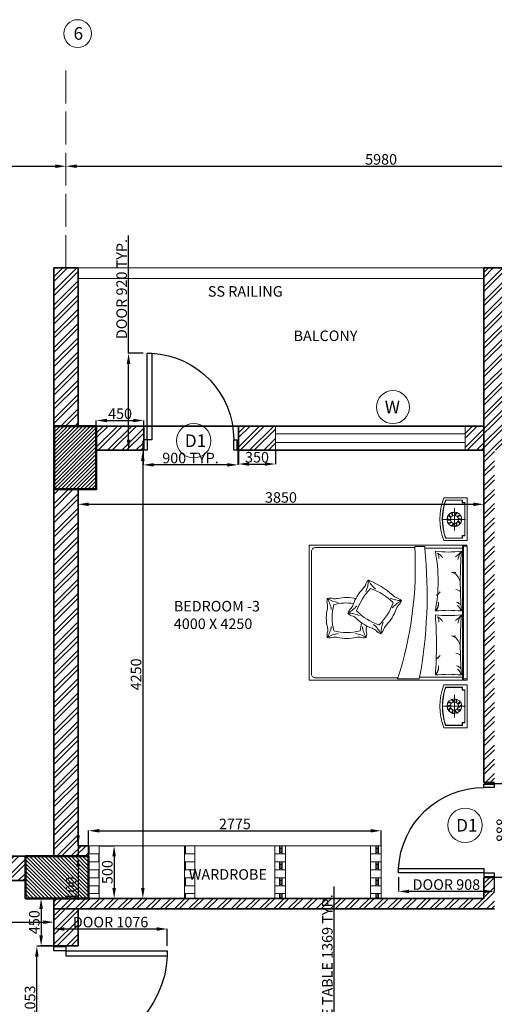
# Model space of a CAD drawing. Units: millimetres. Extents: x -3326 to 29338, y -16792 to 6002.
# Tile 19 of 21: x 16958 to 21462, y -3388 to 5950. Entities that reach past the tile are written whole.
import ezdxf

# ---------------------------------------------------------------- set-up
doc = ezdxf.new("R2010")
doc.units = ezdxf.units.MM
doc.header["$PDMODE"] = 35
doc.header["$PDSIZE"] = 5
doc.linetypes.add('ACAD_ISO04W100', pattern=[30, 24, -3, 0, -3])
for name, color, linetype, lineweight in [('A-ANNO-DIMS', 2, 'Continuous', 13), ('A-ANNO-SYMB', 7, 'Continuous', 18), ('A-AREA-IDEN', 7, 'Continuous', 18), ('A-COLS', 1, 'Continuous', 50), ('A-COLS-PATT', 251, 'Continuous', 13), ('A-DOOR', 3, 'Continuous', 25), ('A-FLOR-CASE', 30, 'Continuous', 18), ('A-FLOR-CASE-PATT', 252, 'Continuous', 13), ('A-FLOR-RAIL', 8, 'Continuous', 20), ('A-GLAZ', 4, 'Continuous', 18), ('A-GRID', 8, 'ACAD_ISO04W100', 13), ('A-GRID-IDEN', 7, 'Continuous', 18), ('A-WALL', 7, 'Continuous', 35), ('A-WALL-PATT', 252, 'Continuous', 13), ('furn', 28, 'Continuous', 18), ('txt', 7, 'Continuous', 18)]:
    doc.layers.add(name, color=color, linetype=linetype, lineweight=lineweight)
doc.styles.get("Standard").update_dxf_attribs({"font": 'arial.ttf'})
doc.dimstyles.new('ISO-25', dxfattribs={"dimtxt": 100, "dimasz": 100, "dimexe": 1.25, "dimexo": 0.625, "dimtad": 1, "dimtxsty": 'Standard', "dimcen": 2.5, "dimadec": 0, "dimazin": 0, "dimtfac": 1, "dimtmove": 0, "dimatfit": 3, "dimfxl": 1, "dimarcsym": 0})
pattern_1 = [(45, (-10476.65, 1e-12), (-67.35192, 67.35192), []), (45, (-10431.74, 1e-12), (-67.35192, 67.35192), [])]

# ---------------------------------------------------------------- blocks, each defined once
blk = doc.blocks.new('A$C0CE462CD')
for p, q in [((860, 100), (860, 0)), ((860, 0), (893.9, 0))]:
    blk.add_line(p, q)
for points in [[(860, 100), (860, 920), (818.4, 920), (818.4, 100)], [(0, 10), (6.1, 10), (6.1, 90), (0, 90)], [(893.9, 10), (900, 10), (900, 90), (893.9, 90)]]:
    blk.add_lwpolyline(points, close=True)
for points in [[(6.1, 0), (40, 0), (40, 100), (6.1, 100)], [(6.1, 100), (6.1, 0)], [(860, 100), (893.9, 100), (893.9, 0)]]:
    blk.add_lwpolyline(points)
blk.add_arc((859.1, 101.9), 819.1, 92.8508, 180.13091)
blk = doc.blocks.new('*D50')
at = {"layer": 'A-ANNO-DIMS', "color": 0, "lineweight": -2, "transparency": 16777216}
for p, q in [((11382.3, -2608.3), (11382.3, -2607.7)), ((11482.3, -2609), (17182.3, -2609)), ((17282.3, -2608.3), (17282.3, -2607.7))]:
    blk.add_line(p, q, dxfattribs=at)
at = {"layer": 'A-ANNO-DIMS', "color": 0, "transparency": 16777216}
for points in [[(11482.3, -2592.3), (11482.3, -2625.6), (11382.3, -2609)], [(17182.3, -2592.3), (17182.3, -2625.6), (17282.3, -2609)]]:
    blk.add_solid(points, dxfattribs=at)
at = {"layer": 'Defpoints', "color": 0, "transparency": 16777216}
for p in [(11382.3, -2609), (17282.3, -2609), (17282.3, -2609)]:
    blk.add_point(p, dxfattribs=at)
at = {"layer": 'A-ANNO-DIMS', "color": 0, "transparency": 16777216, "insert": (14332.3, -2557.3), "char_height": 100, "attachment_point": 5}
blk.add_mtext('5900', dxfattribs=at)
blk = doc.blocks.new('*D52')
at = {"layer": 'A-ANNO-DIMS', "color": 0, "lineweight": -2, "transparency": 16777216}
for p, q in [((17281.7, -2384), (17160, -2384)), ((17161.3, -2484), (17161.3, -2734)), ((17281.7, -2834), (17160, -2834))]:
    blk.add_line(p, q, dxfattribs=at)
at = {"layer": 'A-ANNO-DIMS', "color": 0, "transparency": 16777216}
for points in [[(17144.6, -2484), (17177.9, -2484), (17161.3, -2384)], [(17144.6, -2734), (17177.9, -2734), (17161.3, -2834)]]:
    blk.add_solid(points, dxfattribs=at)
at = {"layer": 'Defpoints', "color": 0, "transparency": 16777216}
for p in [(17282.3, -2384), (17161.3, -2834), (17282.3, -2834)]:
    blk.add_point(p, dxfattribs=at)
at = {"layer": 'A-ANNO-DIMS', "color": 0, "transparency": 16777216, "insert": (17109.6, -2609), "char_height": 100, "attachment_point": 5, "rotation": 90}
blk.add_mtext('450', dxfattribs=at)
blk = doc.blocks.new('*D54')
at = {"layer": 'A-ANNO-DIMS', "color": 0, "lineweight": -2, "transparency": 16777216}
for p, q in [((17512.3, -1784), (17512.3, -1684)), ((17512.3, -1884), (17512.3, -1984)), ((17512.9, -1884), (17513.6, -1884)), ((17512.9, -1984), (17513.6, -1984)), ((17512.3, -2084), (17512.3, -2396.4))]:
    blk.add_line(p, q, dxfattribs=at)
at = {"layer": 'A-ANNO-DIMS', "color": 0, "transparency": 16777216}
for points in [[(17495.6, -1784), (17529, -1784), (17512.3, -1884)], [(17495.6, -2084), (17529, -2084), (17512.3, -1984)]]:
    blk.add_solid(points, dxfattribs=at)
at = {"layer": 'Defpoints', "color": 0, "transparency": 16777216}
for p in [(17512.3, -1884), (17512.3, -1984), (17512.3, -1984)]:
    blk.add_point(p, dxfattribs=at)
at = {"layer": 'A-ANNO-DIMS', "color": 0, "transparency": 16777216, "insert": (17460.6, -2290.2), "char_height": 100, "attachment_point": 5, "rotation": 90}
blk.add_mtext('100', dxfattribs=at)
blk = doc.blocks.new('*D115')
at = {"layer": 'A-ANNO-DIMS', "color": 0, "lineweight": -2, "transparency": 16777216}
for p, q in [((17685, 2096.7), (17685, 2150)), ((17785, 2148.7), (18035, 2148.7)), ((18135, 2096.7), (18135, 2150))]:
    blk.add_line(p, q, dxfattribs=at)
at = {"layer": 'A-ANNO-DIMS', "color": 0, "transparency": 16777216}
for points in [[(17785, 2165.4), (17785, 2132.1), (17685, 2148.7)], [(18035, 2165.4), (18035, 2132.1), (18135, 2148.7)]]:
    blk.add_solid(points, dxfattribs=at)
at = {"layer": 'Defpoints', "color": 0, "transparency": 16777216}
for p in [(18135, 2148.7), (17685, 2096), (18135, 2096)]:
    blk.add_point(p, dxfattribs=at)
at = {"layer": 'A-ANNO-DIMS', "color": 0, "transparency": 16777216, "insert": (17910, 2200.4), "char_height": 100, "attachment_point": 5}
blk.add_mtext('450', dxfattribs=at)
blk = doc.blocks.new('*D116')
at = {"layer": 'A-ANNO-DIMS', "color": 0, "lineweight": -2, "transparency": 16777216}
for p, q in [((19035, 1865.4), (19035, 1734.6)), ((19385, 1865.4), (19385, 1734.6)), ((19135, 1735.9), (19285, 1735.9))]:
    blk.add_line(p, q, dxfattribs=at)
at = {"layer": 'A-ANNO-DIMS', "color": 0, "transparency": 16777216}
for points in [[(19135, 1752.5), (19135, 1719.2), (19035, 1735.9)], [(19285, 1752.5), (19285, 1719.2), (19385, 1735.9)]]:
    blk.add_solid(points, dxfattribs=at)
at = {"layer": 'Defpoints', "color": 0, "transparency": 16777216}
for p in [(19035, 1866), (19385, 1866), (19385, 1735.9)]:
    blk.add_point(p, dxfattribs=at)
at = {"layer": 'A-ANNO-DIMS', "color": 0, "transparency": 16777216, "insert": (19210, 1787.6), "char_height": 100, "attachment_point": 5}
blk.add_mtext('350', dxfattribs=at)
blk = doc.blocks.new('*D117')
at = {"layer": 'A-ANNO-DIMS', "color": 0, "lineweight": -2, "transparency": 16777216}
for p, q in [((17512.3, 1176.9), (17512.3, 1355.4)), ((17612.3, 1354.2), (21262.3, 1354.2)), ((21362.3, 1354.8), (21362.3, 1355.4))]:
    blk.add_line(p, q, dxfattribs=at)
at = {"layer": 'A-ANNO-DIMS', "color": 0, "transparency": 16777216}
for points in [[(17612.3, 1370.8), (17612.3, 1337.5), (17512.3, 1354.2)], [(21262.3, 1370.8), (21262.3, 1337.5), (21362.3, 1354.2)]]:
    blk.add_solid(points, dxfattribs=at)
at = {"layer": 'Defpoints', "color": 0, "transparency": 16777216}
for p in [(21362.3, 1354.2), (21362.3, 1354.2), (17512.3, 1176.3)]:
    blk.add_point(p, dxfattribs=at)
at = {"layer": 'A-ANNO-DIMS', "color": 0, "transparency": 16777216, "insert": (19437.3, 1405.9), "char_height": 100, "attachment_point": 5}
blk.add_mtext('3850', dxfattribs=at)
blk = doc.blocks.new('*D118')
at = {"layer": 'A-ANNO-DIMS', "color": 0, "lineweight": -2, "transparency": 16777216}
for p, q in [((18127.2, 1866), (18127.9, 1866)), ((18126.6, 1766), (18126.6, -2284)), ((18127.2, -2384), (18127.9, -2384))]:
    blk.add_line(p, q, dxfattribs=at)
at = {"layer": 'A-ANNO-DIMS', "color": 0, "transparency": 16777216}
for points in [[(18109.9, 1766), (18143.3, 1766), (18126.6, 1866)], [(18109.9, -2284), (18143.3, -2284), (18126.6, -2384)]]:
    blk.add_solid(points, dxfattribs=at)
at = {"layer": 'Defpoints', "color": 0, "transparency": 16777216}
for p in [(18126.6, 1866), (18126.6, -2384), (18126.6, -2384)]:
    blk.add_point(p, dxfattribs=at)
at = {"layer": 'A-ANNO-DIMS', "color": 0, "transparency": 16777216, "insert": (18074.9, -259), "char_height": 100, "attachment_point": 5, "rotation": 90}
blk.add_mtext('4250', dxfattribs=at)
blk = doc.blocks.new('*D119')
at = {"layer": 'A-ANNO-DIMS', "color": 0, "lineweight": -2, "transparency": 16777216}
for p, q in [((17612.3, -1883.3), (17612.3, -1740.9)), ((17712.3, -1742.2), (20287.3, -1742.2)), ((20387.3, -1883.3), (20387.3, -1740.9))]:
    blk.add_line(p, q, dxfattribs=at)
at = {"layer": 'A-ANNO-DIMS', "color": 0, "transparency": 16777216}
for points in [[(17712.3, -1725.5), (17712.3, -1758.8), (17612.3, -1742.2)], [(20287.3, -1725.5), (20287.3, -1758.8), (20387.3, -1742.2)]]:
    blk.add_solid(points, dxfattribs=at)
at = {"layer": 'Defpoints', "color": 0, "transparency": 16777216}
for p in [(20387.3, -1742.2), (17612.3, -1884), (20387.3, -1884)]:
    blk.add_point(p, dxfattribs=at)
at = {"layer": 'A-ANNO-DIMS', "color": 0, "transparency": 16777216, "insert": (18999.8, -1690.5), "char_height": 100, "attachment_point": 5}
blk.add_mtext('2775', dxfattribs=at)
blk = doc.blocks.new('*D120')
at = {"layer": 'A-ANNO-DIMS', "color": 0, "lineweight": -2, "transparency": 16777216}
for p, q in [((17712.9, -1884), (17855.4, -1884)), ((17854.2, -1984), (17854.2, -2284)), ((17712.9, -2384), (17855.4, -2384))]:
    blk.add_line(p, q, dxfattribs=at)
at = {"layer": 'A-ANNO-DIMS', "color": 0, "transparency": 16777216}
for points in [[(17837.5, -1984), (17870.8, -1984), (17854.2, -1884)], [(17837.5, -2284), (17870.8, -2284), (17854.2, -2384)]]:
    blk.add_solid(points, dxfattribs=at)
at = {"layer": 'Defpoints', "color": 0, "transparency": 16777216}
for p in [(17712.3, -1884), (17712.3, -2384), (17854.2, -2384)]:
    blk.add_point(p, dxfattribs=at)
at = {"layer": 'A-ANNO-DIMS', "color": 0, "transparency": 16777216, "insert": (17802.5, -2134), "char_height": 100, "attachment_point": 5, "rotation": 90}
blk.add_mtext('500', dxfattribs=at)
blk = doc.blocks.new('*D154')
at = {"layer": 'A-ANNO-DIMS', "color": 0, "lineweight": -2, "transparency": 16777216}
for p, q in [((11267.3, 4562.4), (11267.3, 4559.3)), ((11367.3, 4560.5), (17297.3, 4560.5)), ((17397.3, 4561.1), (17397.3, 4561.8))]:
    blk.add_line(p, q, dxfattribs=at)
at = {"layer": 'A-ANNO-DIMS', "color": 0, "transparency": 16777216}
for points in [[(11367.3, 4577.2), (11367.3, 4543.8), (11267.3, 4560.5)], [(17297.3, 4577.2), (17297.3, 4543.8), (17397.3, 4560.5)]]:
    blk.add_solid(points, dxfattribs=at)
at = {"layer": 'Defpoints', "color": 0, "transparency": 16777216}
for p in [(11267.3, 4563), (17397.3, 4560.5), (17397.3, 4560.5)]:
    blk.add_point(p, dxfattribs=at)
at = {"layer": 'A-ANNO-DIMS', "color": 0, "transparency": 16777216, "insert": (14332.3, 4612.2), "char_height": 100, "attachment_point": 5}
blk.add_mtext('6130', dxfattribs=at)
blk = doc.blocks.new('*D155')
at = {"layer": 'A-ANNO-DIMS', "color": 0, "lineweight": -2, "transparency": 16777216}
for p, q in [((17397.3, 4561.1), (17397.3, 4561.8)), ((17497.3, 4560.5), (23277.3, 4560.5)), ((23377.3, 4561.1), (23377.3, 4561.8))]:
    blk.add_line(p, q, dxfattribs=at)
at = {"layer": 'A-ANNO-DIMS', "color": 0, "transparency": 16777216}
for points in [[(17497.3, 4577.2), (17497.3, 4543.8), (17397.3, 4560.5)], [(23277.3, 4577.2), (23277.3, 4543.8), (23377.3, 4560.5)]]:
    blk.add_solid(points, dxfattribs=at)
at = {"layer": 'Defpoints', "color": 0, "transparency": 16777216}
for p in [(17397.3, 4560.5), (23377.3, 4560.5), (23377.3, 4560.5)]:
    blk.add_point(p, dxfattribs=at)
at = {"layer": 'A-ANNO-DIMS', "color": 0, "transparency": 16777216, "insert": (20387.3, 4612.2), "char_height": 100, "attachment_point": 5}
blk.add_mtext('5980', dxfattribs=at)
blk = doc.blocks.new('BED-WITH-NIGHTSTANDS')
for p, q in [((1378.9, 2083.2), (1378.9, 1869.8)), ((1272.3, 1976.5), (1485.6, 1976.5)), ((1466.8, 1702.3), (1097.4, 1702.3)), ((1455.8, 1708.6), (1455.8, 473.4)), ((1466.8, 480.5), (1049.3, 480.5)), ((1378.9, 98.8), (1378.9, 312.2)), ((1272.2, 205.5), (1485.6, 205.5))]:
    blk.add_line(p, q)
for points in [[(1279.5, 2182), (1501.4, 2182), (1501.4, 1775.2), (1279.5, 1775.2, -0.181818)], [(1097.4, 1719.6), (1097.4, 1702.3, -0.072944), (1045.8, 463.1), (840.6, 463.1, 0.092568), (1003.3, 1719.6)], [(1198.4, 1674.1, 0.058596), (1445.6, 1674.1, 0.036889), (1445.6, 1107.7, 0.052163), (1198.4, 1107.7, 0.093111)], [(1198.4, 1070.9, 0.058596), (1445.6, 1070.9, 0.036648), (1445.6, 500.8, 0.052163), (1198.4, 500.8, 0.036967)], [(1279.6, 0), (1501.5, 0), (1501.5, 406.8), (1279.6, 406.8, 0.181818)]]:
    blk.add_lwpolyline(points, format="xyb", close=True)
for points in [[(1454.8, 1797.4), (1295, 1797.4, -0.167087), (1295, 2159.8), (1454.8, 2159.8)], [(1454.8, 1799.6), (1296.6, 1799.6, -0.165559), (1296.6, 2157.6), (1454.8, 2157.6)], [(1003.9, 1708.6), (59.2, 1708.6, 0.414214), (22.2, 1671.6), (22.2, 510.4, 0.414214), (59.2, 473.4), (844.2, 473.4)], [(540, 1293.1, 0.091296), (562.8, 1401.4, 0.091296), (630.7, 1314.1, 0.091296)], [(583.2, 1320, 0.111006), (451.8, 1108.7, 0.119549), (665.6, 975.5, 0.107813), (797.5, 1186.1)], [(797.2, 1187.3, 0.121865), (583.2, 1319.9, 0.121865)], [(211.2, 1122.2, 0.091296), (173.3, 1226.2, 0.091296), (277.2, 1187.9, 0.091296)], [(768.3, 1228.3, 0.091296), (876.7, 1205.8, 0.091296), (789.5, 1137.6, 0.091296)], [(233.7, 1167.8, 0.111006), (234, 919, 0.119549), (485.8, 919, 0.033212), (497.4, 995.5)], [(475.6, 1065.1, 0.091296), (367.2, 1087.5, 0.091296), (454.4, 1155.8)], [(367.2, 1087.5, 0.159461), (418, 1058.9, -0.076283), (449.6, 1036.2, 0.115075), (598.7, 943.3, -0.076283), (633, 924.9, 0.159461), (681.1, 892)], [(277.2, 894.6, 0.091296), (173.3, 856.3, 0.091296), (211.2, 960.3)], [(505.3, 960.3, 0.091296), (543.2, 856.3, 0.091296), (439.3, 894.6, 0.091296)], [(703.9, 1000.2, 0.091296), (681.1, 892, 0.091296), (613.2, 979.3, 0.091296)], [(173.3, 856.3, 0.159461), (231.6, 858.9, -0.076283), (270.5, 856.3, 0.115075), (446, 856.3, -0.076283), (484.9, 858.9, 0.159461), (543.2, 856.3)], [(1454.9, 384.6), (1295.1, 384.6, 0.167087), (1295.1, 22.2), (1454.9, 22.2)], [(1454.9, 382.4), (1296.7, 382.4, 0.165559), (1296.7, 24.4), (1454.9, 24.4)]]:
    blk.add_lwpolyline(points, format="xyb")
for points in [[(1479.2, 2133.2), (1452.6, 2133.2), (1452.6, 2159.8)], [(1479.2, 2135.4), (1454.8, 2135.4), (1454.8, 2159.8)], [(1477, 2135.4), (1477, 1821.8)], [(1479.2, 2135.4), (1479.2, 1821.8)], [(1479.2, 1824), (1452.6, 1824), (1452.6, 1797.4)], [(1479.2, 1821.8), (1454.8, 1821.8), (1454.8, 1797.4)], [(1501.5, 1730.8), (0, 1730.8), (0, 451.2), (1501.5, 451.2)], [(1501.5, 463.1), (1466.8, 463.1), (1466.8, 1723.4), (1501.5, 1723.4), (1501.5, 451.2)], [(1479.3, 358), (1452.7, 358), (1452.7, 384.6)], [(1479.3, 360.2), (1454.9, 360.2), (1454.9, 384.6)], [(1477.1, 46.6), (1477.1, 360.2)], [(1479.3, 46.6), (1479.3, 360.2)], [(1479.3, 48.8), (1452.7, 48.8), (1452.7, 22.2)], [(1479.3, 46.6), (1454.9, 46.6), (1454.9, 22.2)]]:
    blk.add_lwpolyline(points)
for centre, radius in [((1378.9, 1976.5), 69.7), ((1378.9, 1976.5), 37.8), ((1378.9, 205.5), 69.7), ((1378.9, 205.5), 37.8)]:
    blk.add_circle(centre, radius)
for centre, radius, start, end in [((1340.3, 2012.2), 44.8, 226.17003, 272.48975), ((1338.5, 2008.1), 34.1, 214.30017, 274.53802), ((1368.7, 2028), 44.8, 190.17003, 236.48975), ((1364.8, 2025.8), 34.1, 178.30017, 238.53802), ((1400.9, 2024.2), 44.8, 154.17003, 200.48975), ((1396.5, 2024.6), 34.1, 142.30017, 202.53802), ((1424.8, 2002.2), 44.8, 118.17003, 164.48975), ((1421.4, 2005.1), 34.1, 106.30017, 166.53802), ((1431.1, 1970.3), 44.8, 82.17003, 128.48975), ((1430.1, 1974.7), 34.1, 70.30017, 130.53802), ((1389.2, 1925), 44.8, 10.17003, 56.48975), ((1417.5, 1940.8), 44.8, 46.17003, 92.48975), ((1419.3, 1944.9), 34.1, 34.30017, 94.53802), ((1327.7, 1978.3), 34.1, 250.30017, 310.53802), ((1326.7, 1982.7), 44.8, 262.17003, 308.48975), ((1336.4, 1947.9), 34.1, 286.30017, 346.53802), ((1333.1, 1950.8), 44.8, 298.17003, 344.48975), ((1361.4, 1928.3), 34.1, 322.30017, 22.53802), ((1356.9, 1928.8), 44.8, 334.17003, 20.48975), ((1393, 1927.2), 34.1, 358.30017, 58.53802), ((1478, 1708.6), 22.2, 90, 180), ((1175.6, 1619.4), 56.2, 346.48229, 38.55627), ((1192.7, 1576.7), 82.2, 24.2916, 70.9896), ((1214.5, 1859.4), 296.3, 306.49353, 321.27919), ((1652.3, 1542.6), 244.9, 147.53791, 167.5233), ((626.3, 1332.5), 93.8, 132.65224, 168.89294), ((256.3, 651.7), 810, 48.38179, 67.76439), ((1375.3, 1532.7), 61.4, 245.89274, 286.11919), ((1299.1, 1354.7), 137.1, 6.68493, 58.3182), ((785.6, 1046.2), 386.5, 135.13065, 161.38844), ((419.7, 1408.4), 128.4, 315.77185, 333.2208), ((1377, 1216.1), 96.2, 51.81741, 79.89867), ((263.7, 1201.2), 93.8, 164.57915, 200.81985), ((198.5, 1135.9), 93.8, 69.36661, 105.60731), ((242.7, 1351.6), 128.4, 265.03874, 282.4877), ((358.2, 849.8), 386.5, 76.87111, 103.12889), ((884.1, 1348.9), 128.4, 225.58539, 243.03435), ((807.5, 1142.5), 93.8, 42.46578, 78.70648), ((1208.9, 1279), 20.7, 263.75428, 347.21866), ((1026.5, 1507.4), 308.8, 306.20852, 315.08491), ((550.3, 1042.5), 386.5, 167.05756, 193.31535), ((48.2, 1156.4), 128.4, 347.69876, 5.14771), ((360.8, 659.2), 524.3, 83.19556, 104.02838), ((468.2, 1051.5), 107.3, 128.77541, 160.35713), ((298.1, 1211.9), 128.4, 323.29829, 340.74724), ((460, 1247.6), 386.5, 315.13065, 341.38844), ((947.4, 1081.9), 128.4, 143.29829, 160.74724), ((789.7, 1230.6), 90.5, 307.29372, 344.09733), ((1127.7, 1179.9), 101.1, 314.40604, 6.83423), ((1163, 1161), 64, 303.63488, 0.84559), ((1363.4, 1094.5), 103.5, 40.53543, 70.35581), ((1276.2, 1030), 186.4, 24.64565, 44.15848), ((1175.6, 1016.2), 56.2, 346.48229, 38.55627), ((1192.7, 973.5), 82.2, 24.2916, 70.9896), ((1214.5, 1256.2), 296.3, 306.49353, 321.27919), ((1652.3, 939.4), 244.9, 147.53791, 167.5233), ((48.9, 925.3), 128.4, 355.2252, 12.67415), ((669.5, 927.3), 128.4, 167.69876, 185.14771), ((167.4, 1041.2), 386.5, 347.05756, 348.7033), ((626.1, 958.8), 86.6, 309.47264, 349.6505), ((825.9, 885.4), 128.4, 135.77185, 153.2208), ((278.1, 879.2), 107.3, 160.70232, 192.28404), ((461.1, 884), 86.6, 341.39955, 21.57741), ((1375.3, 929.5), 61.4, 245.89274, 286.11919), ((1299.1, 751.6), 137.1, 6.68493, 58.3182), ((1208.9, 675.8), 20.7, 263.75428, 347.21866), ((1026.5, 904.2), 308.8, 306.20852, 315.08491), ((1377, 612.9), 96.2, 51.81741, 79.89867), ((1127.7, 576.7), 101.1, 314.40604, 6.83423), ((1363.4, 491.3), 103.5, 40.53543, 70.35581), ((1163, 557.8), 64, 303.63488, 0.84559), ((1276.2, 426.8), 186.4, 24.64565, 44.15848), ((1478, 473.4), 22.2, 180, 270), ((1340.3, 169.8), 44.8, 87.51025, 133.82997), ((1338.5, 173.9), 34.1, 85.46198, 145.69983), ((1327.7, 203.7), 34.1, 49.46198, 109.69983), ((1326.7, 199.3), 44.8, 51.51025, 97.82997), ((1368.6, 154), 44.8, 123.51025, 169.82997), ((1336.4, 234.2), 34.1, 13.46198, 73.69983), ((1333, 231.2), 44.8, 15.51025, 61.82997), ((1361.4, 253.7), 34.1, 337.46198, 37.69983), ((1356.9, 253.2), 44.8, 339.51025, 25.82997), ((1393, 254.8), 34.1, 301.46198, 1.69983), ((1389.2, 257.1), 44.8, 303.51025, 349.82997), ((1417.5, 241.2), 44.8, 267.51025, 313.82997), ((1419.3, 237.1), 34.1, 265.46198, 325.69983), ((1364.8, 156.2), 34.1, 121.46198, 181.69983), ((1402.8, 152.7), 44.8, 159.51025, 205.82997), ((1398.4, 152.3), 34.1, 157.46198, 217.69983), ((1426.7, 174.7), 44.8, 195.51025, 241.82997), ((1423.3, 171.8), 34.1, 193.46198, 253.69983), ((1433, 206.6), 44.8, 231.51025, 277.82997), ((1430.1, 207.3), 34.1, 229.46198, 289.69983)]:
    blk.add_arc(centre, radius, start, end)
blk = doc.blocks.new('TAG-D1')
blk.add_circle((163.3, 163.3), 163.3)
at = {"insert": (78, 223.5), "char_height": 120, "attachment_point": 1}
blk.add_mtext_dynamic_manual_height_columns('D1', width=137.943, gutter_width=12.5, heights=[0], dxfattribs=at)
blk = doc.blocks.new('TAG-W')
blk.add_circle((156.8, 156.8), 156.8)
at = {"insert": (79.7, 216.8), "char_height": 120, "attachment_point": 1}
blk.add_mtext_dynamic_manual_height_columns('W', width=376.575, gutter_width=12.5, heights=[0], dxfattribs=at)
blk = doc.blocks.new('GLAZ-1800x80')
for p, q in [((0, 80), (1800, 80)), ((0, 0), (1800, 0))]:
    blk.add_line(p, q)
blk = doc.blocks.new('*D183')
at = {"layer": 'A-ANNO-DIMS', "color": 0, "lineweight": -2, "transparency": 16777216}
for p, q in [((17990.9, 2786), (17990.9, 3904.7)), ((18128.3, 2786), (17989.7, 2786)), ((17990.9, 1966), (17990.9, 2686)), ((18128.3, 1866), (17989.7, 1866))]:
    blk.add_line(p, q, dxfattribs=at)
at = {"layer": 'A-ANNO-DIMS', "color": 0, "transparency": 16777216}
for points in [[(17974.3, 2686), (18007.6, 2686), (17990.9, 2786)], [(17974.3, 1966), (18007.6, 1966), (17990.9, 1866)]]:
    blk.add_solid(points, dxfattribs=at)
at = {"layer": 'Defpoints', "color": 0, "transparency": 16777216}
for p in [(17990.9, 2786), (18128.9, 2786), (18128.9, 1866)]:
    blk.add_point(p, dxfattribs=at)
at = {"layer": 'A-ANNO-DIMS', "color": 0, "transparency": 16777216, "insert": (17938.6, 3395.4), "char_height": 100, "attachment_point": 5, "rotation": 90}
blk.add_mtext('DOOR 920 TYP.', dxfattribs=at)
blk = doc.blocks.new('*D184')
at = {"layer": 'A-ANNO-DIMS', "color": 0, "lineweight": -2, "transparency": 16777216}
for p, q in [((18128.9, 1865.4), (18128.9, 1726.8)), ((19028.9, 1865.4), (19028.9, 1726.8)), ((18928.9, 1728), (18228.9, 1728))]:
    blk.add_line(p, q, dxfattribs=at)
at = {"layer": 'A-ANNO-DIMS', "color": 0, "transparency": 16777216}
for points in [[(18228.9, 1744.7), (18228.9, 1711.4), (18128.9, 1728)], [(18928.9, 1744.7), (18928.9, 1711.4), (19028.9, 1728)]]:
    blk.add_solid(points, dxfattribs=at)
at = {"layer": 'Defpoints', "color": 0, "transparency": 16777216}
for p in [(18128.9, 1866), (19028.9, 1866), (18128.9, 1728)]:
    blk.add_point(p, dxfattribs=at)
at = {"layer": 'A-ANNO-DIMS', "color": 0, "transparency": 16777216, "insert": (18578.9, 1779.7), "char_height": 100, "attachment_point": 5}
blk.add_mtext('900 TYP.', dxfattribs=at)
blk = doc.blocks.new('*D187')
at = {"layer": 'A-ANNO-DIMS', "color": 0, "lineweight": -2, "transparency": 16777216}
for p, q in [((20552.7, -2182), (20552.7, -2318.8)), ((21460.8, -2182), (21460.8, -2318.8)), ((21360.8, -2317.6), (20652.7, -2317.6))]:
    blk.add_line(p, q, dxfattribs=at)
at = {"layer": 'A-ANNO-DIMS', "color": 0, "transparency": 16777216}
for points in [[(20652.7, -2300.9), (20652.7, -2334.2), (20552.7, -2317.6)], [(21360.8, -2300.9), (21360.8, -2334.2), (21460.8, -2317.6)]]:
    blk.add_solid(points, dxfattribs=at)
at = {"layer": 'Defpoints', "color": 0, "transparency": 16777216}
for p in [(20552.7, -2181.3), (21460.8, -2181.3), (20552.7, -2317.6)]:
    blk.add_point(p, dxfattribs=at)
at = {"layer": 'A-ANNO-DIMS', "color": 0, "transparency": 16777216, "insert": (21006.8, -2265.2), "char_height": 100, "attachment_point": 5}
blk.add_mtext('DOOR 908', dxfattribs=at)
blk = doc.blocks.new('*D188')
at = {"layer": 'A-ANNO-DIMS', "color": 0, "lineweight": -2, "transparency": 16777216}
for p, q in [((21461.4, -1293), (21598.3, -1293)), ((21597, -1393), (21597, -2081.3)), ((21461.4, -2181.3), (21598.3, -2181.3))]:
    blk.add_line(p, q, dxfattribs=at)
at = {"layer": 'A-ANNO-DIMS', "color": 0, "transparency": 16777216}
for points in [[(21580.4, -1393), (21613.7, -1393), (21597, -1293)], [(21580.4, -2081.3), (21613.7, -2081.3), (21597, -2181.3)]]:
    blk.add_solid(points, dxfattribs=at)
at = {"layer": 'Defpoints', "color": 0, "transparency": 16777216}
for p in [(21460.8, -1293), (21460.8, -2181.3), (21597, -2181.3)]:
    blk.add_point(p, dxfattribs=at)
at = {"layer": 'A-ANNO-DIMS', "color": 0, "transparency": 16777216, "insert": (21545.3, -1737.2), "char_height": 100, "attachment_point": 5, "rotation": 90}
blk.add_mtext('888', dxfattribs=at)
blk = doc.blocks.new('*D193')
at = {"layer": 'A-ANNO-DIMS', "color": 0, "lineweight": -2, "transparency": 16777216}
for p, q in [((17282.3, -2834.6), (17282.3, -2672.5)), ((17382.3, -2673.7), (18258.6, -2673.7)), ((18358.6, -2834.6), (18358.6, -2672.5))]:
    blk.add_line(p, q, dxfattribs=at)
at = {"layer": 'A-ANNO-DIMS', "color": 0, "transparency": 16777216}
for points in [[(17382.3, -2657.1), (17382.3, -2690.4), (17282.3, -2673.7)], [(18258.6, -2657.1), (18258.6, -2690.4), (18358.6, -2673.7)]]:
    blk.add_solid(points, dxfattribs=at)
at = {"layer": 'Defpoints', "color": 0, "transparency": 16777216}
for p in [(18358.6, -2673.7), (17282.3, -2835.2), (18358.6, -2835.2)]:
    blk.add_point(p, dxfattribs=at)
at = {"layer": 'A-ANNO-DIMS', "color": 0, "transparency": 16777216, "insert": (17820.4, -2621.4), "char_height": 100, "attachment_point": 5}
blk.add_mtext('DOOR 1076', dxfattribs=at)
blk = doc.blocks.new('*D194')
at = {"layer": 'A-ANNO-DIMS', "color": 0, "lineweight": -2, "transparency": 16777216}
for p, q in [((17281.7, -2835.2), (17119.6, -2835.2)), ((17120.9, -3788.1), (17120.9, -2935.2)), ((17281.7, -3888.1), (17119.6, -3888.1))]:
    blk.add_line(p, q, dxfattribs=at)
at = {"layer": 'A-ANNO-DIMS', "color": 0, "transparency": 16777216}
for points in [[(17104.2, -2935.2), (17137.5, -2935.2), (17120.9, -2835.2)], [(17104.2, -3788.1), (17137.5, -3788.1), (17120.9, -3888.1)]]:
    blk.add_solid(points, dxfattribs=at)
at = {"layer": 'Defpoints', "color": 0, "transparency": 16777216}
for p in [(17120.9, -2835.2), (17282.3, -2835.2), (17282.3, -3888.1)]:
    blk.add_point(p, dxfattribs=at)
at = {"layer": 'A-ANNO-DIMS', "color": 0, "transparency": 16777216, "insert": (17069.1, -3361.6), "char_height": 100, "attachment_point": 5, "rotation": 90}
blk.add_mtext('1053', dxfattribs=at)
blk = doc.blocks.new('*D229')
at = {"layer": 'A-ANNO-DIMS', "color": 0, "lineweight": -2, "transparency": 16777216}
for p, q in [((19942.4, -4100.4), (19942.4, -2271.4)), ((19737.7, -4100.4), (19943.6, -4100.4)), ((19942.4, -5369), (19942.4, -4200.4)), ((19737.7, -5469), (19943.6, -5469))]:
    blk.add_line(p, q, dxfattribs=at)
at = {"layer": 'A-ANNO-DIMS', "color": 0, "transparency": 16777216}
for points in [[(19925.7, -4200.4), (19959, -4200.4), (19942.4, -4100.4)], [(19925.7, -5369), (19959, -5369), (19942.4, -5469)]]:
    blk.add_solid(points, dxfattribs=at)
at = {"layer": 'Defpoints', "color": 0, "transparency": 16777216}
for p in [(19737.1, -4100.4), (19942.4, -4100.4), (19737.1, -5469)]:
    blk.add_point(p, dxfattribs=at)
at = {"layer": 'A-ANNO-DIMS', "color": 0, "transparency": 16777216, "insert": (19890, -3135.9), "char_height": 100, "attachment_point": 5, "rotation": 90}
blk.add_mtext('COFFEE TABLE 1369 TYP.', dxfattribs=at)

msp = doc.modelspace()

# ---------------------------------------------------------------- hatches: boundary and pattern name
at = {"layer": 'A-COLS-PATT'}
h = msp.add_hatch(dxfattribs=at)
h.set_pattern_fill('ANSI31', color=256, scale=8)
h.set_pattern_definition([(45, (-24436.277, 8703.052), (-17.960512, 17.960512), [])])
h.paths.add_polyline_path([(17285.023, 1496.048), (17685.023, 1496.048), (17685.023, 2096.048), (17285.023, 2096.048)])
h = msp.add_hatch(dxfattribs=at)
h.set_pattern_fill('ANSI31', color=256, scale=8, angle=-90)
h.set_pattern_definition([(315, (24219.305, 39737.347), (17.960512, 17.960512), [])])
h.paths.add_polyline_path([(17012.301, -1983.952), (17012.301, -2383.952), (17612.301, -2383.952), (17612.301, -1983.952)])
at = {"layer": 'A-FLOR-CASE-PATT'}
h = msp.add_hatch(dxfattribs=at)
h.set_pattern_fill('BRSTONE', color=256, scale=9)
h.set_pattern_definition([(0, (-10476.645, 1e-12), (0, 75.438), []), (90, (-10270.9, 1e-12), (-114.3, 75.438), [75.438, -75.438]), (90, (-10293.77, 1e-12), (-114.3, 75.438), [75.438, -75.438]), (0, (-10270.905, 12.57), (114.3, 75.438), [-205.74, 22.86]), (0, (-10270.905, 25.146), (114.3, 75.438), [-205.74, 22.86]), (0, (-10270.905, 37.72), (114.3, 75.438), [-205.74, 22.86]), (0, (-10270.905, 50.29), (114.3, 75.438), [-205.74, 22.86]), (0, (-10270.905, 62.865), (114.3, 75.438), [-205.74, 22.86])])
h.paths.add_polyline_path([(17712.301, -1883.952), (17612.301, -1883.952), (17612.301, -1983.952), (17612.301, -2383.952), (17712.301, -2383.952)])
h.paths.add_polyline_path([(18620.634, -1883.952), (18520.634, -1883.952), (18520.634, -2383.952), (18620.634, -2383.952)])
h.paths.add_polyline_path([(19478.967, -1883.952), (19378.967, -1883.952), (19378.967, -2383.952), (19478.967, -2383.952)])
h.paths.add_polyline_path([(20387.301, -1883.952), (20287.301, -1883.952), (20287.301, -2383.952), (20387.301, -2383.952)])
at = {"layer": 'A-WALL-PATT'}
h = msp.add_hatch(dxfattribs=at)
h.set_pattern_fill('ANSI32', color=256, scale=10)
h.set_pattern_definition(pattern_1)
h.paths.add_polyline_path([(12212.301, -1983.952), (11640.861, -1983.952), (11640.861, -2213.952), (12212.301, -2213.952)])
h.paths.add_polyline_path([(14712.301, -1983.952), (14012.301, -1983.952), (14012.301, -2213.952), (14712.301, -2213.952)])
h.paths.add_polyline_path([(17012.301, -1983.952), (16512.301, -1983.952), (16512.301, -2213.952), (17012.301, -2213.952)])
h.paths.add_polyline_path([(11382.301, -2383.952), (11040.861, -2383.952), (7302.301, -2383.952), (7302.301, -1935.766), (7217.026, -1935.766), (7202.301, -1933.952), (7202.301, -2483.952), (7302.301, -2483.952), (11152.301, -2483.952), (11152.301, -2833.952), (11283.549, -2833.952), (11283.549, -2830.395), (11363.875, -2830.395), (11382.301, -2833.952)])
h.paths.add_polyline_path([(11382.301, -3733.952), (11363.875, -3733.952), (11363.875, -3734.058), (11283.549, -3734.058), (11152.301, -3733.952), (11152.301, -6450.401), (11382.301, -6450.401)])
h.paths.add_polyline_path([(13462.301, -6450.401), (12606.738, -6450.401), (11382.301, -6450.401), (11382.301, -6680.401), (12606.738, -6680.401), (13462.301, -6680.401)])
h.paths.add_polyline_path([(11382.301, -7050.401), (11152.301, -7050.401), (11152.301, -8810.401), (11382.301, -8810.401)])
h.paths.add_polyline_path([(13462.301, -8980.401), (11751.174, -8980.401), (11751.174, -9210.401), (13462.301, -9210.401)])
h.paths.add_polyline_path([(13962.301, -6850.401), (13732.301, -6850.401), (13732.301, -7350.401), (13962.301, -7350.401)])
h.paths.add_polyline_path([(13962.301, -8309.482), (13732.301, -8309.482), (13732.301, -8809.482), (13962.301, -8809.482)])
h.paths.add_polyline_path([(15712.301, -12533.952), (12902.301, -12533.952), (12902.301, -12763.952), (15712.301, -12763.952)])
h.paths.add_polyline_path([(11508.301, -9211.585), (11382.301, -9211.585), (11152.301, -9211.585), (11152.301, -11033.952), (10952.301, -11033.952), (10952.301, -11263.952), (11152.301, -11263.952), (11152.301, -12361.585), (11508.301, -12361.585)])
h.paths.add_polyline_path([(12002.301, -12533.952), (11902.301, -12533.952), (11902.301, -12761.585), (11152.301, -12761.585), (11152.301, -12763.952), (11902.301, -12763.952), (12002.301, -12763.952)])
h.paths.add_polyline_path([(17112.301, -12533.952), (16912.301, -12533.952), (16912.301, -12763.952), (17112.301, -12763.952)])
h.paths.add_polyline_path([(11382.301, 3596.048), (11152.301, 3596.048), (11152.301, 2096.048), (11382.301, 2096.048)])
h.paths.add_polyline_path([(11382.301, 1496.048), (11152.301, 1496.048), (11152.301, -1983.952), (11382.301, -1983.952)])
h = msp.add_hatch(dxfattribs=at)
h.set_pattern_fill('ANSI32', color=256, scale=10)
h.set_pattern_definition(pattern_1)
h.paths.add_polyline_path([(29282.301, -7283.952), (28882.301, -7283.952), (28882.301, -7383.952), (29052.301, -7383.952), (29052.301, -10763.952), (29282.301, -10763.952)])
h.paths.add_polyline_path([(29282.301, -11263.952), (29052.301, -11263.952), (29052.301, -12763.952), (29282.301, -12763.952)])
h.paths.add_polyline_path([(25052.301, -11263.952), (25652.301, -11263.952), (25652.301, -11123.904), (25652.289, -11123.904), (25652.289, -11033.952), (25052.301, -11033.952), (24572.301, -11033.952), (24572.301, -11263.952), (24822.301, -11263.952), (24822.301, -12763.952), (25052.301, -12763.952)])
h.paths.add_polyline_path([(26902.301, -11033.952), (26552.301, -11033.952), (26552.301, -11263.952), (26902.301, -11263.952)])
h.paths.add_polyline_path([(21992.301, -6683.952), (21362.301, -6683.952), (17512.301, -6683.952), (17512.301, -6783.952), (21362.301, -6783.952), (21992.301, -6783.952)])
h.paths.add_polyline_path([(17512.301, -7283.952), (17282.301, -7283.952), (17282.301, -12163.952), (17512.301, -12163.952), (17512.301, -11263.952), (18112.301, -11263.952), (18112.301, -11033.952), (17512.301, -11033.952)])
h.paths.add_polyline_path([(21462.301, -8211.864), (21462.064, -8211.864), (21462.064, -8142.609), (21462.301, -8133.952), (21362.301, -8133.952), (21362.301, -8233.952), (21362.301, -11033.952), (21162.301, -11033.952), (21162.301, -11263.952), (21362.301, -11263.952), (21362.301, -12763.952), (21592.301, -12763.952), (21592.301, -11263.952), (21992.301, -11263.952), (21992.301, -11033.952), (21592.301, -11033.952), (21462.301, -11033.952)])
h.paths.add_polyline_path([(24152.301, -8133.952), (23322.301, -8133.952), (23322.301, -7433.952), (23092.301, -7433.952), (23092.301, -8133.952), (22241.021, -8133.952), (22241.021, -8142.609), (22241.182, -8142.609), (22241.182, -8211.864), (22241.021, -8233.952), (23092.301, -8233.952), (23092.301, -10513.206), (23322.301, -10513.206), (23322.301, -8233.952), (24152.301, -8233.952)])
h.paths.add_polyline_path([(25052.301, -8233.952), (25052.301, -8133.952), (24952.301, -8133.952), (24952.301, -11033.952), (25052.301, -11033.952)])
h.paths.add_polyline_path([(23972.301, -11033.952), (23493.251, -11033.952), (23493.251, -11263.952), (23972.301, -11263.952)])
h.paths.add_polyline_path([(23092.301, -11033.952), (22592.301, -11033.952), (22592.301, -11263.952), (23092.301, -11263.952)])
h.paths.add_polyline_path([(28882.301, -11033.952), (28702.301, -11033.952), (28702.301, -11263.952), (28882.301, -11263.952)])
h.paths.add_polyline_path([(17512.301, -3883.952), (17387.589, -3883.952), (17387.589, -3888.07), (17282.301, -3888.07), (17282.301, -6683.952), (17512.301, -6683.952)])
h.paths.add_polyline_path([(21462.301, -2183.952), (21362.301, -2183.952), (21362.301, -2383.952), (17282.301, -2383.952), (17282.301, -2483.952), (17512.301, -2483.952), (21462.301, -2483.952)])
h.paths.add_polyline_path([(17512.301, -2483.952), (17282.301, -2483.952), (17282.301, -2833.952), (17512.301, -2833.952)])
h.paths.add_polyline_path([(21462.301, 1866.048), (21992.301, 1866.048), (21992.301, 2096.048), (21592.301, 2096.048), (21592.301, 3596.048), (21362.301, 3596.048), (21362.301, 1866.048), (21362.301, -1283.952), (21462.301, -1283.952)])
h.paths.add_polyline_path([(17512.301, 1496.048), (17282.301, 1496.048), (17282.301, -1983.952), (17612.301, -1983.952), (17612.301, -1883.952), (17512.301, -1883.952)])
h.paths.add_polyline_path([(17512.301, 3596.048), (17282.301, 3596.048), (17282.301, 2096.048), (17512.301, 2096.048)])
h.paths.add_polyline_path([(18135.023, 2096.048), (17685.023, 2096.048), (17685.023, 1866.048), (18135.023, 1866.048), (18135.023, 1876.048), (18128.942, 1876.048), (18128.942, 1956.048), (18135.023, 1956.048)])
h.paths.add_polyline_path([(19385.023, 2096.048), (19035.023, 2096.048), (19035.023, 1866.048), (19385.023, 1866.048)])
h.paths.add_polyline_path([(21362.301, 2096.048), (21185.023, 2096.048), (21185.023, 1866.048), (21362.301, 1866.048)])
h.paths.add_polyline_path([(23092.301, 2096.048), (22592.301, 2096.048), (22592.301, 1866.048), (23092.301, 1866.048)])
h.paths.add_polyline_path([(23972.301, 2096.048), (23492.301, 2096.048), (23492.301, 1866.048), (23972.301, 1866.048)])
h.paths.add_polyline_path([(23972.301, 2496.048), (23872.301, 2496.048), (23872.301, 2096.048), (23972.301, 2096.048)])
h.paths.add_polyline_path([(22692.301, 2496.048), (22592.301, 2496.048), (22592.301, 2096.048), (22692.301, 2096.048)])
h.paths.add_polyline_path([(23322.301, 1346.048), (23092.301, 1346.048), (23092.301, -1733.952), (23322.301, -1733.952)])
h.paths.add_polyline_path([(23092.301, -933.952), (22262.301, -933.952), (22262.301, -1033.952), (23092.301, -1033.952)])
h.paths.add_polyline_path([(24952.301, -1433.952), (24952.301, -1733.952), (23492.301, -1733.952), (23492.301, -1833.952), (24952.301, -1833.952), (24952.301, -2483.952), (25052.301, -2483.952), (25052.301, -2466.23), (25049.26, -2466.23), (25049.26, -2386.23), (25049.941, -1433.952)])
h.paths.add_polyline_path([(22692.301, -11263.952), (22592.301, -11263.952), (22592.301, -11663.952), (22692.301, -11663.952)])
h.paths.add_polyline_path([(23972.301, -11263.952), (23872.301, -11263.952), (23872.301, -11663.952), (23972.301, -11663.952)])

# ---------------------------------------------------------------- linework, layer by layer
at = {"layer": 'A-COLS'}
for points in [[(17285.023, 2096.048), (17685.023, 2096.048), (17685.023, 1496.048), (17285.023, 1496.048)], [(17612.301, -1983.952), (17612.301, -2383.952), (17012.301, -2383.952), (17012.301, -1983.952)]]:
    msp.add_lwpolyline(points, close=True, dxfattribs=at)
at = {"layer": 'A-FLOR-CASE'}
for p, q in [((17612.301, -1883.952), (17712.301, -1883.952)), ((17712.301, -1883.952), (17712.301, -2383.952)), ((17712.301, -1883.952), (20287.301, -1883.952)), ((18520.634, -1883.952), (18520.634, -2383.952)), ((18620.634, -1883.952), (18620.634, -2383.952)), ((19378.967, -1883.952), (19378.967, -2383.952)), ((19478.967, -1883.952), (19478.967, -2383.952)), ((20287.301, -1883.952), (20287.301, -2383.952)), ((20287.301, -1883.952), (20387.301, -1883.952)), ((20387.301, -1883.952), (20387.301, -2383.952)), ((17612.301, -1983.952), (17612.301, -2383.952))]:
    msp.add_line(p, q, dxfattribs=at)
at = {"layer": 'A-FLOR-RAIL'}
for p, q in [((21362.301, 3596.048), (17512.301, 3596.048)), ((21362.301, 3496.048), (17512.301, 3496.048))]:
    msp.add_line(p, q, dxfattribs=at)
at = {"layer": 'A-GLAZ'}
for p, q in [((19385.023, 2096.048), (19385.023, 1866.048)), ((21185.023, 2096.048), (21185.023, 1866.048))]:
    msp.add_line(p, q, dxfattribs=at)
at = {"layer": 'A-GRID', "ltscale": 13}
msp.add_line((17397.301, 3596.048), (17397.301, 5524.981), dxfattribs=at)
at = {"layer": 'A-GRID-IDEN'}
msp.add_circle((17508.647, 5818.449), 131.628, dxfattribs=at)
at = {"layer": 'A-WALL'}
for p, q in [((17282.301, 3596.048), (17282.301, -1983.952)), ((17512.301, 3596.048), (17282.301, 3596.048)), ((17512.301, 3596.048), (17512.301, 2096.048)), ((21362.301, 3596.048), (21362.301, 1866.048)), ((21592.301, 3596.048), (21362.301, 3596.048)), ((21362.301, 2096.048), (17282.301, 2096.048)), ((18135.023, 2096.048), (18135.023, 1866.048)), ((19035.023, 2096.048), (19035.023, 1866.048)), ((18135.023, 1866.048), (17685.023, 1866.048)), ((21362.301, 1866.048), (19035.023, 1866.048)), ((21362.301, 1866.048), (21362.301, -1283.952)), ((17512.301, 1496.048), (17512.301, -1883.952)), ((21462.301, -1283.952), (21362.301, -1283.952)), ((17612.301, -1883.952), (17512.301, -1883.952)), ((17612.301, -1983.952), (17612.301, -1883.952)), ((17012.301, -1983.952), (11640.861, -1983.952)), ((17012.301, -2213.952), (11640.861, -2213.952)), ((21462.301, -2183.952), (21362.301, -2183.952)), ((21362.301, -2183.952), (21362.301, -2383.952)), ((21362.301, -2383.952), (17282.301, -2383.952)), ((17282.301, -2383.952), (17282.301, -2833.952)), ((17512.301, -2483.952), (17282.301, -2483.952)), ((17512.301, -2483.952), (17512.301, -2833.952)), ((21462.301, -2483.952), (17512.301, -2483.952)), ((17282.301, -2833.952), (17512.301, -2833.952))]:
    msp.add_line(p, q, dxfattribs=at)

# ---------------------------------------------------------------- block references
at = {"layer": 'A-ANNO-SYMB'}
for name, p in [('TAG-W', (20342.788, 2119.007)), ('TAG-D1', (18446.629, 1793.582)), ('TAG-D1', (21020.838, -1853.23))]:
    msp.add_blockref(name, p, dxfattribs=at)
at = {"layer": 'A-DOOR', "xscale": -1}
msp.add_blockref('A$C0CE462CD', (19028.942, 1866.048), dxfattribs=at)
at = {"layer": 'A-DOOR'}
for p, xscale, yscale, zscale, rotation in [((21460.805, -1292.986), -0.9870629254581404, 0.9870629254581404, 0.9870629254581404, 90), ((17282.301, -3888.07), -1.169867667365197, 1.169867667365197, 1.169867667365197, 270)]:
    msp.add_blockref('A$C0CE462CD', p, dxfattribs=dict(at, xscale=xscale, yscale=yscale, zscale=zscale, rotation=rotation))
at = {"layer": 'A-GLAZ'}
msp.add_blockref('GLAZ-1800x80', (19385.023, 1941.048), dxfattribs=at)
at = {"layer": 'furn'}
msp.add_blockref('BED-WITH-NIGHTSTANDS', (19703.523, -765.386), dxfattribs=at)

# ---------------------------------------------------------------- texts
at = {"layer": 'A-AREA-IDEN', "char_height": 100, "attachment_point": 1}
for s, insert in [('BALCONY', (19556.833, 3002.348)), ('BEDROOM -3\\P4000 X 4250', (18420.42, 437.658))]:
    msp.add_mtext_dynamic_manual_height_columns(s, width=1168.90663, gutter_width=12.5, heights=[0], dxfattribs=dict(at, insert=insert))
at = {"layer": 'A-GRID-IDEN', "insert": (17469.029, 5879.718), "char_height": 120, "attachment_point": 1}
msp.add_mtext_dynamic_manual_height_columns('6', width=463.74815, gutter_width=12.5, heights=[120.491], dxfattribs=at)
at = {"layer": 'txt', "char_height": 100, "attachment_point": 1}
for s, insert in [('SS RAILING', (18743.71, 3423.27)), ('WARDROBE', (18562.537, -2106.153))]:
    msp.add_mtext_dynamic_manual_height_columns(s, width=1168.90663, gutter_width=12.5, heights=[0], dxfattribs=dict(at, insert=insert))

# ---------------------------------------------------------------- dimensions: what is measured, and where the dimension line sits
at = {"layer": 'A-ANNO-DIMS'}
for base, p1, p2, picture, middle in [((17397.301, 4560.514), (11267.301, 4563.014), (17397.301, 4560.514), '*D154', (14332.301, 4612.231)), ((23377.301, 4560.514), (17397.301, 4560.514), (23377.301, 4560.514), '*D155', (20387.301, 4612.197)), ((18135.023, 2148.732), (17685.023, 2096.048), (18135.023, 2096.048), '*D115', (17910.023, 2200.415)), ((19385.023, 1735.851), (19035.023, 1866.048), (19385.023, 1866.048), '*D116', (19210.023, 1787.567)), ((21362.301, 1354.161), (17512.301, 1176.251), (21362.301, 1354.161), '*D117', (19437.301, 1405.877)), ((20387.301, -1742.151), (17612.301, -1883.952), (20387.301, -1883.952), '*D119', (18999.801, -1690.469)), ((17282.301, -2608.952), (11382.301, -2608.952), (17282.301, -2608.952), '*D50', (14332.301, -2557.27))]:
    dim = msp.add_linear_dim(base=base, p1=p1, p2=p2, dimstyle='ISO-25', override={"dimclrd": 0, "dimclre": 0, "dimclrt": 0}, dxfattribs=at)
    dim.commit()
    dim.dimension.update_dxf_attribs({"geometry": picture, "text_midpoint": middle})
for base, p1, p2, angle, text, picture, middle in [((17990.942, 2786.048), (18128.942, 1866.048), (18128.942, 2786.048), 90, 'DOOR <> TYP.', '*D183', (17938.577, 3395.37)), ((18128.942, 1728.048), (19028.942, 1866.048), (18128.942, 1866.048), 180, '<> TYP.', '*D184', (18578.942, 1779.73)), ((20552.707, -2317.558), (21460.805, -2181.343), (20552.707, -2181.343), 180, 'DOOR <>', '*D187', (21006.756, -2265.193)), ((19942.36, -4100.372), (19737.067, -5468.994), (19737.067, -4100.372), 90, 'COFFEE TABLE <> TYP.', '*D229', (19889.961, -3135.866))]:
    dim = msp.add_linear_dim(base=base, p1=p1, p2=p2, angle=angle, text=text, dimstyle='ISO-25', override={"dimdec": 0, "dimlfac": 1, "dimrnd": 0, "dimzin": 0, "dimdsep": 46, "dimlunit": 2}, dxfattribs=at)
    dim.commit()
    dim.dimension.update_dxf_attribs({"geometry": picture, "text_midpoint": middle})
for base, p1, p2, angle, override, picture, middle in [((18126.612, -2383.952), (18126.612, 1866.048), (18126.612, -2383.952), 90, {"dimclrd": 0, "dimclre": 0, "dimclrt": 0}, '*D118', (18074.93, -258.952)), ((21597.02, -2181.343), (21460.805, -1292.986), (21460.805, -2181.343), 270, {"dimdec": 0, "dimlfac": 1, "dimrnd": 0, "dimzin": 0, "dimdsep": 46, "dimlunit": 2}, '*D188', (21545.337, -1737.165)), ((17512.301, -1983.952), (17512.301, -1883.952), (17512.301, -1983.952), 90, {"dimclrd": 0, "dimclre": 0, "dimclrt": 0}, '*D54', (17460.618, -2290.171)), ((17854.164, -2383.952), (17712.301, -1883.952), (17712.301, -2383.952), 90, {"dimclrd": 0, "dimclre": 0, "dimclrt": 0}, '*D120', (17802.482, -2133.952)), ((17161.268, -2833.952), (17282.301, -2383.952), (17282.301, -2833.952), 90, {"dimclrd": 0, "dimclre": 0, "dimclrt": 0}, '*D52', (17109.586, -2608.952)), ((17120.859, -2835.189), (17282.301, -3888.07), (17282.301, -2835.189), 90, {"dimdec": 0, "dimlfac": 1, "dimrnd": 0, "dimzin": 0, "dimdsep": 46, "dimlunit": 2}, '*D194', (17069.143, -3361.63))]:
    dim = msp.add_linear_dim(base=base, p1=p1, p2=p2, angle=angle, dimstyle='ISO-25', override=override, dxfattribs=at)
    dim.commit()
    dim.dimension.update_dxf_attribs({"geometry": picture, "text_midpoint": middle})
dim = msp.add_linear_dim(base=(18358.579, -2673.748), p1=(17282.301, -2835.189), p2=(18358.579, -2835.189), text='DOOR <>', dimstyle='ISO-25', override={"dimdec": 0, "dimlfac": 1, "dimrnd": 0, "dimzin": 0, "dimdsep": 46, "dimlunit": 2}, dxfattribs=at)
dim.commit()
dim.dimension.update_dxf_attribs({"geometry": '*D193', "text_midpoint": (17820.44, -2621.383)})

doc.saveas('drawing.dxf')
